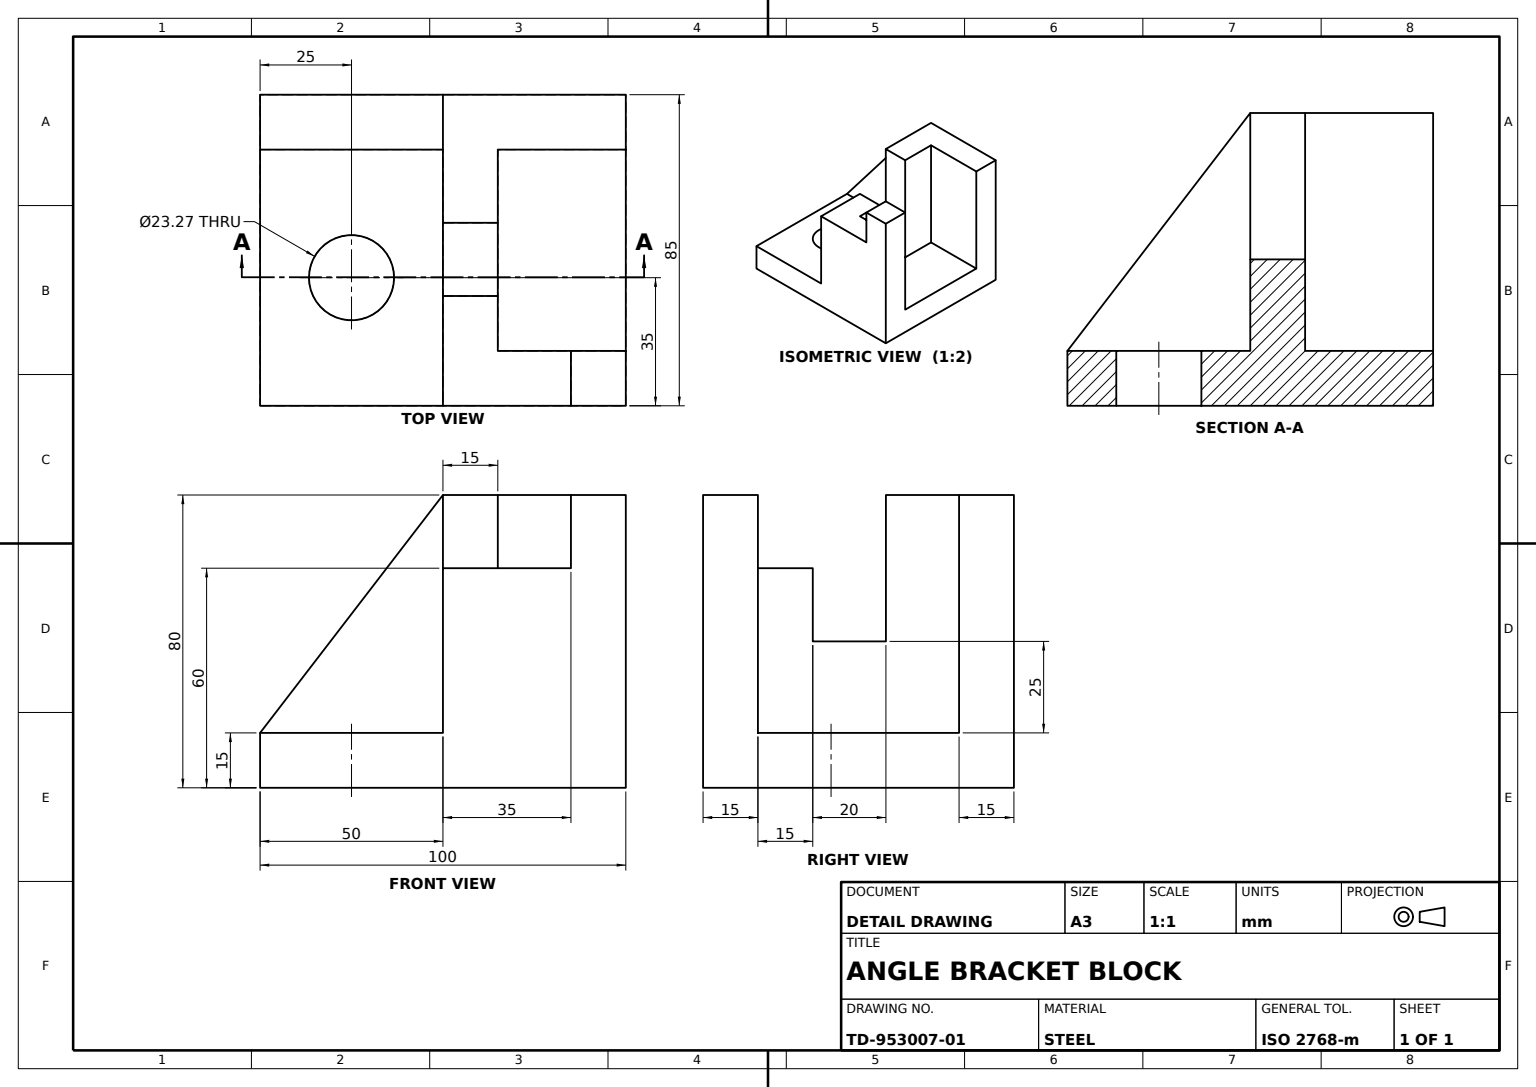
SolidWorks part; units mm, degrees
material "Plain Carbon Steel"
ref_plane "Front Plane" through (0, 0, 0) normal (0, 0, 1) x (1, 0, 0)
ref_plane "Top Plane" through (0, 0, 0) normal (0, 1, 0) x (1, 0, 0)
ref_plane "Right Plane" through (0, 0, 0) normal (1, 0, 0) x (0, 0, -1)
sketch "Base Plate Sketch" plane through (0, 0, 0) normal (0, 1, 0) x (1, 0, 0)
  line L1 (-42.5, -50) -> (42.5, -50)
  line L2 (-42.5, -50) -> (-42.5, 50)
  line L3 (-42.5, 50) -> (42.5, 50)
  line L4 (42.5, -50) -> (42.5, 50)
  line L5 (-42.5, -50) -> (42.5, 50) construction
  line L6 (-42.5, 50) -> (42.5, -50) construction
  point P0 (0, 0)
  dimension "D1" = 100
  dimension "D2" = 85
extrude "Base Plate" add sketch "Base Plate Sketch" along normal blind 15
sketch "Upright Wall Sketch" plane through (42.5, 0, 0) normal (1, 0, 0) x (0, 0, -1)
  line L0 (50, 0) -> (50, 80)
  line L1 (50, 80) -> (35, 80)
  line L2 (35, 80) -> (35, 60)
  line L3 (35, 60) -> (0, 60)
  line L4 (0, 60) -> (0, 15)
  line L5 (-50, 15) -> (50, 15) construction
  line L6 (0, 15) -> (50, 15)
  line M9 (50, 15) -> (-50, 15)
  dimension "D1" = 80
  dimension "D2" = 15
  dimension "D3" = 20
  dimension "D4" = 35
extrude "Upright Wall" add sketch "Upright Wall Sketch" against normal blind 15 contours L3 L4 L0 L1 L2 M9
sketch "Side Wall Sketch" plane through (-42.5, 0, 0) normal (-1, 0, 0) x (0, 0, 1)
  line L0 (-50, 80) -> (0, 80)
  line L1 (0, 80) -> (0, 15)
  line L2 (-50, 15) -> (0, 15) construction
  line L3 (0, 15) -> (-50, 15)
  line L4 (-50, 15) -> (-50, 80)
  line L5 (-50, 15) -> (-50, 80) construction
  dimension "D1" = 50
extrude "Side Wall" add sketch "Side Wall Sketch" against normal blind 15
sketch "Gusset Sketch" plane through (-42.5, 0, 0) normal (-1, 0, 0) x (0, 0, 1)
  line L0 (0, 80) -> (50, 15)
  line L1 (50, 15) -> (0, 15)
  line L2 (0, 15) -> (0, 80)
extrude "Gusset" add sketch "Gusset Sketch" against normal blind 15
sketch "Post Sketch" plane through (0, 80, 0) normal (0, 1, 0) x (1, 0, 0)
  line L0 (-27.5, 0) -> (-7.5, 0)
  line L1 (-7.5, 0) -> (-7.5, 15)
  line L2 (-7.5, 15) -> (-27.5, 15)
  line L3 (-27.5, 50) -> (-27.5, -50) construction
  line L5 (-27.5, 15) -> (-27.5, 0)
  dimension "D1" = 20
  dimension "D2" = 15
extrude "Post" add sketch "Post Sketch" against normal blind 60
sketch "Stepped Block Sketch" plane through (0, 0, 0) normal (0, 0, 1) x (1, 0, 0)
  line L1 (12.5, 40) -> (12.5, 60)
  line L2 (12.5, 60) -> (27.5, 60)
  line L3 (27.5, 60) -> (27.5, 15)
  line L5 (42.5, 60) -> (42.5, 15) construction
  line L9 (12.5, 40) -> (-7.5, 40)
  line L13 (-7.5, 15) -> (27.5, 15)
  line L14 (-7.5, 40) -> (-27.5, 40)
  line L15 (-27.5, 40) -> (-27.5, 14.7909)
  line L16 (-7.5, 15) -> (-27.5, 14.7909)
  dimension "D1" = 15
  dimension "D2" = 20
  dimension "D3" = 70
  dimension "D4" = 45.2091
  dimension "D5" = 20
  dimension "D6" = 25
extrude "Stepped Block" add sketch "Stepped Block Sketch" against normal blind 15
sketch "Mounting Hole Sketch" plane through (0, 15, 0) normal (0, 1, 0) x (1, 0, 0)
  line L0 (42.5, -50) -> (42.5, 0) construction
  line L2 (-27.5, -50) -> (42.5, -50) construction
  circle A0 centre (7.5, -25) radius 11.6364
  dimension "D1" = 35
  dimension "D3" = 23.2728
  dimension "D2" = 25
extrude "Mounting Hole" cut sketch "Mounting Hole Sketch" against normal blind 15
